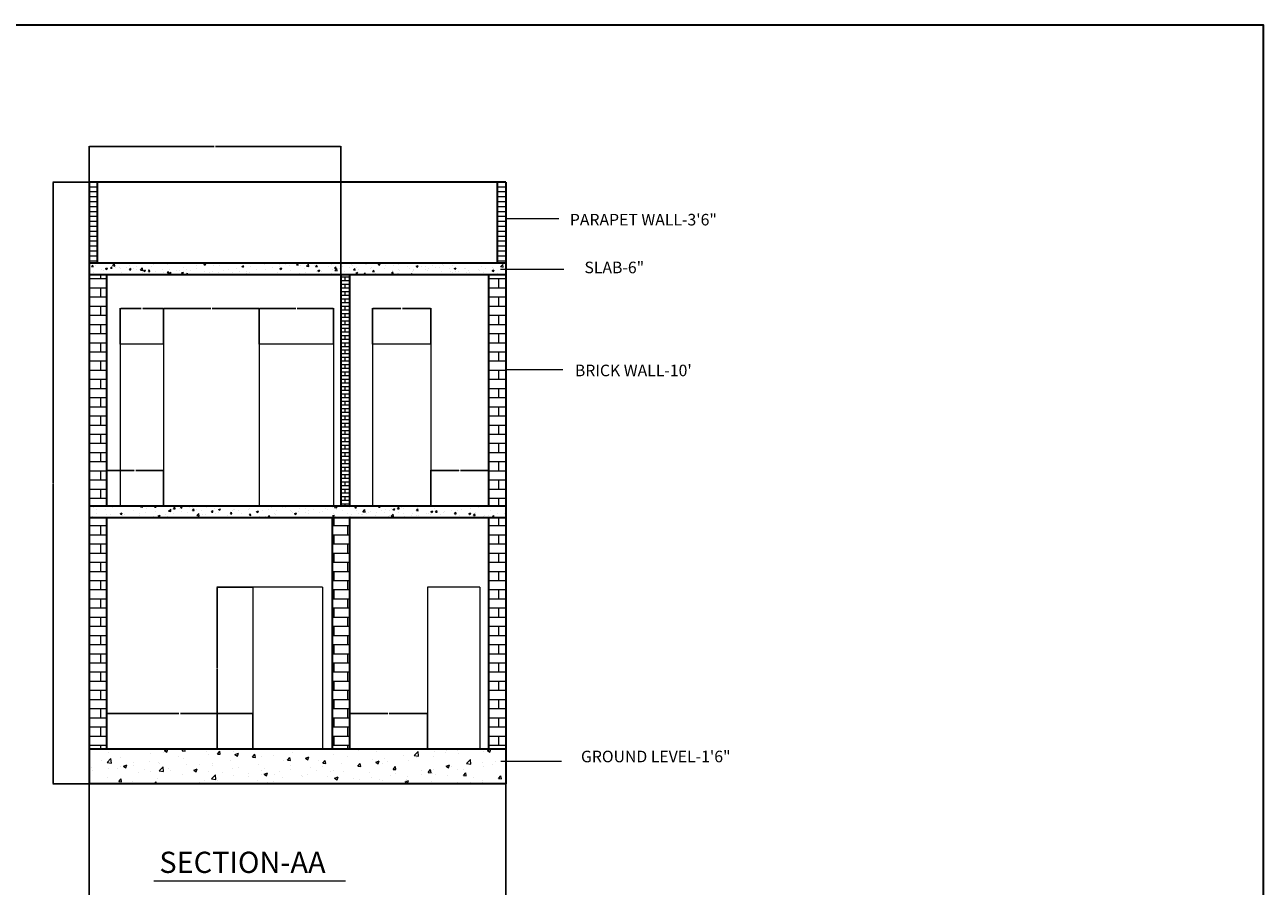
# Model space of a CAD drawing. Units: inches. Extents: x 2003 to 3241, y 1726 to 2849.
# Tile 7 of 7: x 2599 to 3241, y 2402 to 2849. Entities that reach past the tile are written whole.
import ezdxf

# ---------------------------------------------------------------- set-up
doc = ezdxf.new("R2010")
doc.units = ezdxf.units.IN
for name, color, linetype, lineweight in [('A-ANNO-DIMS', 2, 'Continuous', 18), ('A-ANNO-TEXT', 7, 'Continuous', 18), ('A-ANNO-TTLB', 7, 'Continuous', 35), ('A-SECT', 7, 'Continuous', 35), ('A-SECT-BYND', 7, 'Continuous', 18), ('A-SECT-PATT', 252, 'Continuous', 13), ('A-WALL-PATT', 252, 'Continuous', 13)]:
    doc.layers.add(name, color=color, linetype=linetype, lineweight=lineweight)
doc.styles.get("Standard").update_dxf_attribs({"font": 'arial.ttf'})
doc.dimstyles.get("Standard").update_dxf_attribs({"dimtxt": 0.18, "dimasz": 0.18, "dimexe": 0.18, "dimexo": 0.0625, "dimgap": 0.09, "dimtad": 0, "dimtih": 1, "dimtoh": 1, "dimdec": 4, "dimzin": 0, "dimdsep": 46, "dimtxsty": 'Standard', "dimcen": 0.09, "dimadec": 0, "dimazin": 0, "dimtfac": 1, "dimtdec": 4, "dimtofl": 0, "dimtmove": 0, "dimatfit": 3, "dimfxl": 1, "dimtolj": 1, "dimtzin": 0, "dimarcsym": 0})

# ---------------------------------------------------------------- blocks, each defined once
blk = doc.blocks.new('*D100')
at = {"layer": 'A-ANNO-DIMS', "color": 0, "lineweight": -2, "transparency": 16777216}
for p, q in [((2632.44, 2455.12), (2632.44, 2386.37)), ((2848.44, 2455.12), (2848.44, 2386.37)), ((2632.62, 2386.55), (2740.15, 2386.55)), ((2848.26, 2386.55), (2740.73, 2386.55))]:
    blk.add_line(p, q, dxfattribs=at)
at = {"layer": 'A-ANNO-DIMS', "color": 0, "transparency": 16777216}
for points in [[(2632.62, 2386.58), (2632.62, 2386.52), (2632.44, 2386.55)], [(2848.26, 2386.58), (2848.26, 2386.52), (2848.44, 2386.55)]]:
    blk.add_solid(points, dxfattribs=at)
at = {"layer": 'Defpoints', "color": 0, "transparency": 16777216}
for p in [(2632.44, 2455.18), (2848.44, 2455.18), (2848.44, 2386.55)]:
    blk.add_point(p, dxfattribs=at)
at = {"layer": 'A-ANNO-DIMS', "color": 0, "transparency": 16777216, "insert": (2740.44, 2386.55), "char_height": 0.18, "attachment_point": 5}
blk.add_mtext('\\A1;216', dxfattribs=at)
blk = doc.blocks.new('*D101')
at = {"layer": 'A-ANNO-DIMS', "color": 0, "lineweight": -2, "transparency": 16777216}
for p, q in [((2632.38, 2767.18), (2613.76, 2767.18)), ((2613.94, 2767), (2613.94, 2611.36)), ((2613.94, 2455.36), (2613.94, 2611)), ((2632.38, 2455.18), (2613.76, 2455.18))]:
    blk.add_line(p, q, dxfattribs=at)
at = {"layer": 'A-ANNO-DIMS', "color": 0, "transparency": 16777216}
for points in [[(2613.91, 2767), (2613.97, 2767), (2613.94, 2767.18)], [(2613.91, 2455.36), (2613.97, 2455.36), (2613.94, 2455.18)]]:
    blk.add_solid(points, dxfattribs=at)
at = {"layer": 'Defpoints', "color": 0, "transparency": 16777216}
for p in [(2613.94, 2767.18), (2632.44, 2767.18), (2632.44, 2455.18)]:
    blk.add_point(p, dxfattribs=at)
at = {"layer": 'A-ANNO-DIMS', "color": 0, "transparency": 16777216, "insert": (2613.94, 2611.18), "char_height": 0.18, "attachment_point": 5}
blk.add_mtext('\\A1;312', dxfattribs=at)
blk = doc.blocks.new('*D102')
at = {"layer": 'A-ANNO-DIMS', "color": 0, "lineweight": -2, "transparency": 16777216}
for p, q in [((2632.44, 2719.24), (2632.44, 2785.86)), ((2632.62, 2785.68), (2697.31, 2785.68)), ((2762.76, 2785.68), (2698.08, 2785.68)), ((2762.94, 2719.24), (2762.94, 2785.86))]:
    blk.add_line(p, q, dxfattribs=at)
at = {"layer": 'A-ANNO-DIMS', "color": 0, "transparency": 16777216}
for points in [[(2632.62, 2785.71), (2632.62, 2785.65), (2632.44, 2785.68)], [(2762.76, 2785.71), (2762.76, 2785.65), (2762.94, 2785.68)]]:
    blk.add_solid(points, dxfattribs=at)
at = {"layer": 'Defpoints', "color": 0, "transparency": 16777216}
for p in [(2762.94, 2785.68), (2632.44, 2719.18), (2762.94, 2719.18)]:
    blk.add_point(p, dxfattribs=at)
at = {"layer": 'A-ANNO-DIMS', "color": 0, "transparency": 16777216, "insert": (2697.69, 2785.68), "char_height": 0.18, "attachment_point": 5}
blk.add_mtext('\\A1;130.5', dxfattribs=at)
blk = doc.blocks.new('*D103')
at = {"layer": 'A-ANNO-DIMS', "color": 0, "lineweight": -2, "transparency": 16777216}
for p, q in [((2641.44, 2473.24), (2641.44, 2491.86)), ((2641.62, 2491.68), (2679.01, 2491.68)), ((2717.18, 2491.68), (2679.79, 2491.68)), ((2717.36, 2473.24), (2717.36, 2491.86))]:
    blk.add_line(p, q, dxfattribs=at)
at = {"layer": 'A-ANNO-DIMS', "color": 0, "transparency": 16777216}
for points in [[(2641.62, 2491.71), (2641.62, 2491.65), (2641.44, 2491.68)], [(2717.18, 2491.71), (2717.18, 2491.65), (2717.36, 2491.68)]]:
    blk.add_solid(points, dxfattribs=at)
at = {"layer": 'Defpoints', "color": 0, "transparency": 16777216}
for p in [(2717.36, 2491.68), (2641.44, 2473.18), (2717.36, 2473.18)]:
    blk.add_point(p, dxfattribs=at)
at = {"layer": 'A-ANNO-DIMS', "color": 0, "transparency": 16777216, "insert": (2679.4, 2491.68), "char_height": 0.18, "attachment_point": 5}
blk.add_mtext('\\A1;75.92', dxfattribs=at)
blk = doc.blocks.new('*D104')
at = {"layer": 'A-ANNO-DIMS', "color": 0, "lineweight": -2, "transparency": 16777216}
for p, q in [((2767.44, 2473.24), (2767.44, 2491.86)), ((2767.62, 2491.68), (2787.36, 2491.68)), ((2807.76, 2491.68), (2788.02, 2491.68)), ((2807.94, 2473.24), (2807.94, 2491.86))]:
    blk.add_line(p, q, dxfattribs=at)
at = {"layer": 'A-ANNO-DIMS', "color": 0, "transparency": 16777216}
for points in [[(2767.62, 2491.71), (2767.62, 2491.65), (2767.44, 2491.68)], [(2807.76, 2491.71), (2807.76, 2491.65), (2807.94, 2491.68)]]:
    blk.add_solid(points, dxfattribs=at)
at = {"layer": 'Defpoints', "color": 0, "transparency": 16777216}
for p in [(2807.94, 2491.68), (2767.44, 2473.18), (2807.94, 2473.18)]:
    blk.add_point(p, dxfattribs=at)
at = {"layer": 'A-ANNO-DIMS', "color": 0, "transparency": 16777216, "insert": (2787.69, 2491.68), "char_height": 0.18, "attachment_point": 5}
blk.add_mtext('\\A1;40.5', dxfattribs=at)
blk = doc.blocks.new('*D105')
at = {"layer": 'A-ANNO-DIMS', "color": 0, "lineweight": -2, "transparency": 16777216}
for p, q in [((2717.3, 2557.18), (2698.68, 2557.18)), ((2698.86, 2557), (2698.86, 2515.36)), ((2698.86, 2473.36), (2698.86, 2515)), ((2717.3, 2473.18), (2698.68, 2473.18))]:
    blk.add_line(p, q, dxfattribs=at)
at = {"layer": 'A-ANNO-DIMS', "color": 0, "transparency": 16777216}
for points in [[(2698.83, 2557), (2698.89, 2557), (2698.86, 2557.18)], [(2698.83, 2473.36), (2698.89, 2473.36), (2698.86, 2473.18)]]:
    blk.add_solid(points, dxfattribs=at)
at = {"layer": 'Defpoints', "color": 0, "transparency": 16777216}
for p in [(2698.86, 2557.18), (2717.36, 2557.18), (2717.36, 2473.18)]:
    blk.add_point(p, dxfattribs=at)
at = {"layer": 'A-ANNO-DIMS', "color": 0, "transparency": 16777216, "insert": (2698.86, 2515.18), "char_height": 0.18, "attachment_point": 5}
blk.add_mtext('\\A1;84', dxfattribs=at)
blk = doc.blocks.new('*D106')
at = {"layer": 'A-ANNO-DIMS', "color": 0, "lineweight": -2, "transparency": 16777216}
for p, q in [((2641.44, 2599.24), (2641.44, 2617.86)), ((2641.62, 2617.68), (2655.88, 2617.68)), ((2670.92, 2617.68), (2656.67, 2617.68)), ((2671.1, 2599.24), (2671.1, 2617.86))]:
    blk.add_line(p, q, dxfattribs=at)
at = {"layer": 'A-ANNO-DIMS', "color": 0, "transparency": 16777216}
for points in [[(2641.62, 2617.71), (2641.62, 2617.65), (2641.44, 2617.68)], [(2670.92, 2617.71), (2670.92, 2617.65), (2671.1, 2617.68)]]:
    blk.add_solid(points, dxfattribs=at)
at = {"layer": 'Defpoints', "color": 0, "transparency": 16777216}
for p in [(2671.1, 2617.68), (2641.44, 2599.18), (2671.1, 2599.18)]:
    blk.add_point(p, dxfattribs=at)
at = {"layer": 'A-ANNO-DIMS', "color": 0, "transparency": 16777216, "insert": (2656.27, 2617.68), "char_height": 0.18, "attachment_point": 5}
blk.add_mtext('\\A1;29.66', dxfattribs=at)
blk = doc.blocks.new('*D107')
at = {"layer": 'A-ANNO-DIMS', "color": 0, "lineweight": -2, "transparency": 16777216}
for p, q in [((2648.67, 2683.24), (2648.67, 2701.86)), ((2648.85, 2701.68), (2659.42, 2701.68)), ((2670.92, 2701.68), (2660.35, 2701.68)), ((2671.1, 2683.24), (2671.1, 2701.86))]:
    blk.add_line(p, q, dxfattribs=at)
at = {"layer": 'A-ANNO-DIMS', "color": 0, "transparency": 16777216}
for points in [[(2648.85, 2701.71), (2648.85, 2701.65), (2648.67, 2701.68)], [(2670.92, 2701.71), (2670.92, 2701.65), (2671.1, 2701.68)]]:
    blk.add_solid(points, dxfattribs=at)
at = {"layer": 'Defpoints', "color": 0, "transparency": 16777216}
for p in [(2671.1, 2701.68), (2648.67, 2683.18), (2671.1, 2683.18)]:
    blk.add_point(p, dxfattribs=at)
at = {"layer": 'A-ANNO-DIMS', "color": 0, "transparency": 16777216, "insert": (2659.89, 2701.68), "char_height": 0.18, "attachment_point": 5}
blk.add_mtext('\\A1;22.434', dxfattribs=at)
blk = doc.blocks.new('*D108')
at = {"layer": 'A-ANNO-DIMS', "color": 0, "lineweight": -2, "transparency": 16777216}
for p, q in [((2671.1, 2683.24), (2671.1, 2701.86)), ((2671.28, 2701.68), (2695.5, 2701.68)), ((2720.52, 2701.68), (2696.3, 2701.68)), ((2720.7, 2683.24), (2720.7, 2701.86))]:
    blk.add_line(p, q, dxfattribs=at)
at = {"layer": 'A-ANNO-DIMS', "color": 0, "transparency": 16777216}
for points in [[(2671.28, 2701.71), (2671.28, 2701.65), (2671.1, 2701.68)], [(2720.52, 2701.71), (2720.52, 2701.65), (2720.7, 2701.68)]]:
    blk.add_solid(points, dxfattribs=at)
at = {"layer": 'Defpoints', "color": 0, "transparency": 16777216}
for p in [(2720.7, 2701.68), (2671.1, 2683.18), (2720.7, 2683.18)]:
    blk.add_point(p, dxfattribs=at)
at = {"layer": 'A-ANNO-DIMS', "color": 0, "transparency": 16777216, "insert": (2695.9, 2701.68), "char_height": 0.18, "attachment_point": 5}
blk.add_mtext('\\A1;49.59', dxfattribs=at)
blk = doc.blocks.new('*D109')
at = {"layer": 'A-ANNO-DIMS', "color": 0, "lineweight": -2, "transparency": 16777216}
for p, q in [((2720.7, 2683.24), (2720.7, 2701.86)), ((2720.88, 2701.68), (2739.58, 2701.68)), ((2759.07, 2701.68), (2740.37, 2701.68)), ((2759.25, 2683.24), (2759.25, 2701.86))]:
    blk.add_line(p, q, dxfattribs=at)
at = {"layer": 'A-ANNO-DIMS', "color": 0, "transparency": 16777216}
for points in [[(2720.88, 2701.71), (2720.88, 2701.65), (2720.7, 2701.68)], [(2759.07, 2701.71), (2759.07, 2701.65), (2759.25, 2701.68)]]:
    blk.add_solid(points, dxfattribs=at)
at = {"layer": 'Defpoints', "color": 0, "transparency": 16777216}
for p in [(2759.25, 2701.68), (2720.7, 2683.18), (2759.25, 2683.18)]:
    blk.add_point(p, dxfattribs=at)
at = {"layer": 'A-ANNO-DIMS', "color": 0, "transparency": 16777216, "insert": (2739.98, 2701.68), "char_height": 0.18, "attachment_point": 5}
blk.add_mtext('\\A1;38.56', dxfattribs=at)
blk = doc.blocks.new('*D110')
at = {"layer": 'A-ANNO-DIMS', "color": 0, "lineweight": -2, "transparency": 16777216}
for p, q in [((2809.63, 2599.24), (2809.63, 2617.86)), ((2809.81, 2617.68), (2824.16, 2617.68)), ((2839.26, 2617.68), (2824.92, 2617.68)), ((2839.44, 2599.24), (2839.44, 2617.86))]:
    blk.add_line(p, q, dxfattribs=at)
at = {"layer": 'A-ANNO-DIMS', "color": 0, "transparency": 16777216}
for points in [[(2809.81, 2617.71), (2809.81, 2617.65), (2809.63, 2617.68)], [(2839.26, 2617.71), (2839.26, 2617.65), (2839.44, 2617.68)]]:
    blk.add_solid(points, dxfattribs=at)
at = {"layer": 'Defpoints', "color": 0, "transparency": 16777216}
for p in [(2839.44, 2617.68), (2809.63, 2599.18), (2839.44, 2599.18)]:
    blk.add_point(p, dxfattribs=at)
at = {"layer": 'A-ANNO-DIMS', "color": 0, "transparency": 16777216, "insert": (2824.54, 2617.68), "char_height": 0.18, "attachment_point": 5}
blk.add_mtext('\\A1;29.81', dxfattribs=at)
blk = doc.blocks.new('*D111')
at = {"layer": 'A-ANNO-DIMS', "color": 0, "lineweight": -2, "transparency": 16777216}
for p, q in [((2779.37, 2683.24), (2779.37, 2701.86)), ((2779.55, 2701.68), (2794.11, 2701.68)), ((2809.45, 2701.68), (2794.9, 2701.68)), ((2809.63, 2683.24), (2809.63, 2701.86))]:
    blk.add_line(p, q, dxfattribs=at)
at = {"layer": 'A-ANNO-DIMS', "color": 0, "transparency": 16777216}
for points in [[(2779.55, 2701.71), (2779.55, 2701.65), (2779.37, 2701.68)], [(2809.45, 2701.71), (2809.45, 2701.65), (2809.63, 2701.68)]]:
    blk.add_solid(points, dxfattribs=at)
at = {"layer": 'Defpoints', "color": 0, "transparency": 16777216}
for p in [(2809.63, 2701.68), (2779.37, 2683.18), (2809.63, 2683.18)]:
    blk.add_point(p, dxfattribs=at)
at = {"layer": 'A-ANNO-DIMS', "color": 0, "transparency": 16777216, "insert": (2794.5, 2701.68), "char_height": 0.18, "attachment_point": 5}
blk.add_mtext('\\A1;30.26', dxfattribs=at)

msp = doc.modelspace()

# ---------------------------------------------------------------- hatches: boundary and pattern name
at = {"layer": 'A-SECT-PATT'}
h = msp.add_hatch(dxfattribs=at)
h.set_pattern_fill('AR-CONC', color=256, scale=0.054, style=0)
h.paths.add_polyline_path([(2632.4427, 2719.181), (2848.4427, 2719.181), (2848.4427, 2725.181), (2632.4427, 2725.181)])
h = msp.add_hatch(dxfattribs=at)
h.set_pattern_fill('AR-CONC', color=256, scale=0.054, style=0)
h.paths.add_polyline_path([(2632.4427, 2593.181), (2848.4427, 2593.181), (2848.4427, 2599.181), (2632.4427, 2599.181)])
h = msp.add_hatch(dxfattribs=at)
h.set_pattern_fill('AR-CONC', color=256, scale=0.1, style=0)
h.paths.add_polyline_path([(2632.4427, 2455.181), (2848.4427, 2455.181), (2848.4427, 2473.181), (2632.4427, 2473.181)])
at = {"layer": 'A-WALL-PATT'}
h = msp.add_hatch(dxfattribs=at)
h.set_pattern_fill('LINE', color=256, scale=0.806299, style=0)
h.paths.add_polyline_path([(2632.4427, 2725.181), (2636.9204, 2725.181), (2636.9204, 2767.181), (2632.4427, 2767.181)])
h = msp.add_hatch(dxfattribs=at)
h.set_pattern_fill('LINE', color=256, scale=0.806299, style=0)
h.paths.add_polyline_path([(2844.1413, 2725.181), (2848.4427, 2725.181), (2848.4427, 2767.181), (2844.1413, 2767.181)])
h = msp.add_hatch(dxfattribs=at)
h.set_pattern_fill('AR-BRSTD', color=256, scale=0.07, style=0)
h.paths.add_polyline_path([(2632.4427, 2599.181), (2641.4427, 2599.181), (2641.4427, 2719.181), (2632.4427, 2719.181)])
h = msp.add_hatch(dxfattribs=at)
h.set_pattern_fill('AR-BRSTD', color=256, scale=0.028, style=0)
h.paths.add_polyline_path([(2762.9427, 2599.181), (2767.4427, 2599.181), (2767.4427, 2719.181), (2762.9427, 2719.181)])
h = msp.add_hatch(dxfattribs=at)
h.set_pattern_fill('AR-BRSTD', color=256, scale=0.07, style=0)
h.paths.add_polyline_path([(2839.4427, 2599.181), (2848.4427, 2599.181), (2848.4427, 2719.181), (2839.4427, 2719.181)])
h = msp.add_hatch(dxfattribs=at)
h.set_pattern_fill('AR-BRSTD', color=256, scale=0.07, style=0)
h.paths.add_polyline_path([(2632.4427, 2473.181), (2641.4427, 2473.181), (2641.4427, 2593.181), (2632.4427, 2593.181)])
h = msp.add_hatch(dxfattribs=at)
h.set_pattern_fill('AR-BRSTD', color=256, scale=0.07, style=0)
h.paths.add_polyline_path([(2758.4427, 2473.181), (2767.4427, 2473.181), (2767.4427, 2593.181), (2758.4427, 2593.181)])
h = msp.add_hatch(dxfattribs=at)
h.set_pattern_fill('AR-BRSTD', color=256, scale=0.07, style=0)
h.paths.add_polyline_path([(2839.4427, 2473.181), (2848.4427, 2473.181), (2848.4427, 2593.181), (2839.4427, 2593.181)])

# ---------------------------------------------------------------- linework, layer by layer
at = {"layer": 'A-ANNO-TEXT'}
for p, q in [((2848.4427, 2748.3659), (2875.9196, 2748.3659)), ((2845.7042, 2721.9953), (2878.5678, 2721.9953)), ((2848.4427, 2670.0661), (2878.1043, 2670.0661)), ((2845.999, 2466.9392), (2877.3848, 2466.9392)), ((2666.0953, 2405.0531), (2765.3634, 2405.0531))]:
    msp.add_line(p, q, dxfattribs=at)
at = {"layer": 'A-ANNO-TTLB'}
msp.add_lwpolyline([(2003.2633, 2848.7261), (3241.1194, 2848.7261), (3241.1194, 1726.227), (2003.2633, 1726.227)], close=True, dxfattribs=at)
at = {"layer": 'A-SECT'}
for p, q in [((2632.4427, 2767.181), (2632.4427, 2581.181)), ((2848.4427, 2767.181), (2632.4427, 2767.181)), ((2636.9204, 2725.181), (2636.9204, 2767.181)), ((2844.1413, 2725.181), (2844.1413, 2767.181)), ((2848.4427, 2767.181), (2848.4427, 2581.181)), ((2848.4427, 2725.181), (2632.4427, 2725.181)), ((2848.4427, 2719.181), (2632.4427, 2719.181)), ((2641.4427, 2719.181), (2641.4427, 2599.181)), ((2762.9427, 2719.181), (2762.9427, 2599.181)), ((2767.4427, 2719.181), (2767.4427, 2599.181)), ((2839.4427, 2719.181), (2839.4427, 2599.181)), ((2632.4427, 2641.181), (2632.4427, 2455.181)), ((2848.4427, 2641.181), (2848.4427, 2455.181)), ((2848.4427, 2599.181), (2632.4427, 2599.181)), ((2848.4427, 2599.181), (2632.4427, 2599.181)), ((2848.4427, 2593.181), (2632.4427, 2593.181)), ((2641.4427, 2593.181), (2641.4427, 2473.181)), ((2758.4427, 2593.181), (2758.4427, 2473.181)), ((2767.4427, 2593.181), (2767.4427, 2473.181)), ((2839.4427, 2593.181), (2839.4427, 2473.181)), ((2848.4427, 2473.181), (2632.4427, 2473.181)), ((2848.4427, 2455.181), (2632.4427, 2455.181))]:
    msp.add_line(p, q, dxfattribs=at)
at = {"layer": 'A-SECT-BYND'}
for p, q in [((2648.6706, 2683.181), (2648.6706, 2599.181)), ((2671.1046, 2683.181), (2648.6706, 2683.181)), ((2671.1046, 2683.181), (2671.1046, 2599.181)), ((2720.6979, 2683.181), (2720.6979, 2599.181)), ((2759.2549, 2683.181), (2720.6979, 2683.181)), ((2759.2549, 2683.181), (2759.2549, 2599.181)), ((2779.3738, 2683.181), (2779.3738, 2599.181)), ((2809.6324, 2683.181), (2779.3738, 2683.181)), ((2809.6324, 2683.181), (2809.6324, 2599.181)), ((2717.3625, 2557.181), (2717.3625, 2473.181)), ((2753.3872, 2557.181), (2717.3625, 2557.181)), ((2753.3872, 2557.181), (2753.3872, 2473.181)), ((2807.9427, 2557.181), (2807.9427, 2473.181)), ((2835.1013, 2557.181), (2807.9427, 2557.181)), ((2835.1013, 2557.181), (2835.1013, 2473.181))]:
    msp.add_line(p, q, dxfattribs=at)

# ---------------------------------------------------------------- texts
at = {"layer": 'A-ANNO-TEXT', "attachment_point": 1}
for s, width, insert, char_height in [('PARAPET WALL-3\'6"', 149.979891, (2881.6947, 2750.695), 6), ('SLAB-6"', 37.932122, (2889.2511, 2725.9206), 6), ("BRICK WALL-10'", 93.630114, (2884.3142, 2672.531), 6), ('GROUND LEVEL-1\'6"', 126.537511, (2887.4621, 2472.4216), 6), ('SECTION-AA', 211.445382, (2668.9066, 2420.0609), 11)]:
    msp.add_mtext_dynamic_manual_height_columns(s, width=width, gutter_width=12.5, heights=[0], dxfattribs=dict(at, insert=insert, char_height=char_height))

# ---------------------------------------------------------------- dimensions: what is measured, and where the dimension line sits
at = {"layer": 'A-ANNO-DIMS'}
for base, p1, p2, override, picture, middle in [((2762.9427, 2785.681), (2632.4427, 2719.181), (2762.9427, 2719.181), {"dimdec": 1, "dimlfac": 1, "dimrnd": 0, "dimzin": 0, "dimdsep": 46, "dimlunit": 2}, '*D102', (2697.6927, 2785.681)), ((2671.1046, 2701.681), (2648.6706, 2683.181), (2671.1046, 2683.181), {"dimdec": 3, "dimlfac": 1, "dimrnd": 0, "dimzin": 0, "dimdsep": 46, "dimlunit": 2}, '*D107', (2659.8876, 2701.681)), ((2720.6979, 2701.681), (2671.1046, 2683.181), (2720.6979, 2683.181), {"dimdec": 2, "dimlfac": 1, "dimrnd": 0, "dimzin": 0, "dimdsep": 46, "dimlunit": 2}, '*D108', (2695.9012, 2701.681)), ((2759.2549, 2701.681), (2720.6979, 2683.181), (2759.2549, 2683.181), {"dimdec": 2, "dimlfac": 1, "dimrnd": 0, "dimzin": 0, "dimdsep": 46, "dimlunit": 2}, '*D109', (2739.9764, 2701.681)), ((2809.6324, 2701.681), (2779.3738, 2683.181), (2809.6324, 2683.181), {"dimdec": 2, "dimlfac": 1, "dimrnd": 0, "dimzin": 0, "dimdsep": 46, "dimlunit": 2}, '*D111', (2794.5031, 2701.681)), ((2671.1046, 2617.681), (2641.4427, 2599.181), (2671.1046, 2599.181), {"dimdec": 2, "dimlfac": 1, "dimrnd": 0, "dimzin": 0, "dimdsep": 46, "dimlunit": 2}, '*D106', (2656.2736, 2617.681)), ((2839.4427, 2617.681), (2809.6324, 2599.181), (2839.4427, 2599.181), {"dimdec": 2, "dimlfac": 1, "dimrnd": 0, "dimzin": 0, "dimdsep": 46, "dimlunit": 2}, '*D110', (2824.5376, 2617.681)), ((2717.3625, 2491.681), (2641.4427, 2473.181), (2717.3625, 2473.181), {"dimdec": 2, "dimlfac": 1, "dimrnd": 0, "dimzin": 0, "dimdsep": 46, "dimlunit": 2}, '*D103', (2679.4026, 2491.681)), ((2807.9427, 2491.681), (2767.4427, 2473.181), (2807.9427, 2473.181), {"dimdec": 1, "dimlfac": 1, "dimrnd": 0, "dimzin": 0, "dimdsep": 46, "dimlunit": 2}, '*D104', (2787.6927, 2491.681)), ((2848.4427, 2386.5531), (2632.4427, 2455.181), (2848.4427, 2455.181), {"dimdec": 0, "dimlfac": 1, "dimrnd": 0, "dimzin": 0, "dimdsep": 46, "dimlunit": 2}, '*D100', (2740.4427, 2386.5531))]:
    dim = msp.add_linear_dim(base=base, p1=p1, p2=p2, dimstyle='Standard', override=override, dxfattribs=at)
    dim.commit()
    dim.dimension.update_dxf_attribs({"geometry": picture, "text_midpoint": middle})
for base, p1, p2, picture, middle in [((2613.9427, 2767.181), (2632.4427, 2455.181), (2632.4427, 2767.181), '*D101', (2613.9427, 2611.181)), ((2698.8625, 2557.181), (2717.3625, 2473.181), (2717.3625, 2557.181), '*D105', (2698.8625, 2515.181))]:
    dim = msp.add_linear_dim(base=base, p1=p1, p2=p2, angle=90, dimstyle='Standard', override={"dimdec": 0, "dimlfac": 1, "dimrnd": 0, "dimzin": 0, "dimdsep": 46, "dimlunit": 2}, dxfattribs=at)
    dim.commit()
    dim.dimension.update_dxf_attribs({"geometry": picture, "text_midpoint": middle})

doc.saveas('drawing.dxf')
